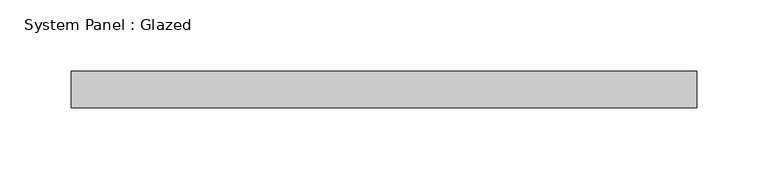
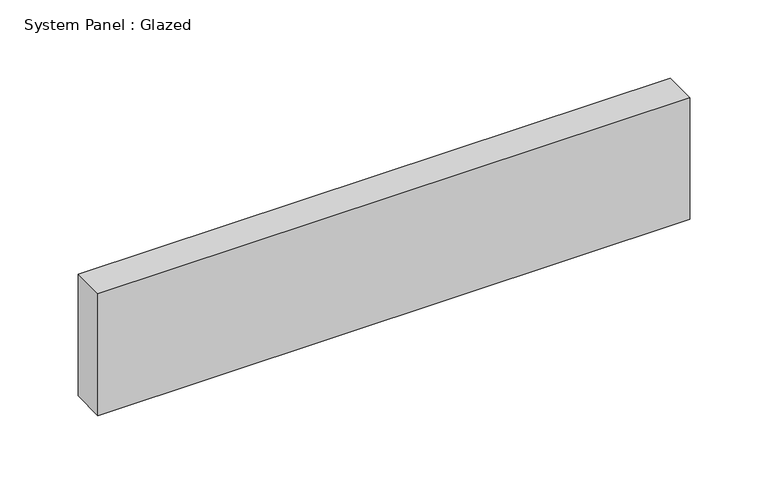
"""IFC4 building model written with IfcOpenShell, lengths in millimetres: plate geometry, System Panel : Glazed."""

from ifc_helpers import new_model, si_unit, origin, origin_with_axes, place, context, project, spatial, polyline, outline, extrude, source, transform, mapped, element, save


def system_panel_glazed_19038302(model_context):
    return source(origin(), model_context, "Body", "SweptSolid", [
        extrude(outline(polyline([(219.075, 19.05), (-219.075, 19.05), (-219.075, 44.45), (219.075, 44.45), (219.075, 19.05)])), origin_with_axes(), (0.0, 0.0, 1.0), 95.25),
    ])


if __name__ == "__main__":
    model = new_model("IFC4")
    model_context = context("Model", 3, world=origin())
    ifc_project = project(units=[si_unit("LENGTHUNIT", "METRE", prefix="MILLI")], contexts=[model_context])
    site = spatial("IfcSite", under=ifc_project)
    building = spatial("IfcBuilding", under=site)
    placement = place(None, origin())
    system_panel_glazed_shape = system_panel_glazed_19038302(model_context)
    element("IfcPlate", 1, ObjectType="System Panel : Glazed", at=placement, inside=building, context=model_context, shape_type="MappedRepresentation", body=[
        mapped(system_panel_glazed_shape, transform((0.0, 0.0, 0.0), x_axis=(1.0, 0.0, 0.0), y_axis=(0.0, 1.0, 0.0), z_axis=(0.0, 0.0, 1.0))),
    ])
    save(model, "model.ifc")

# Revit data of these elements
# Type "System Panel : Glazed"
#   Construction Type Id = "GSP4R"
#   Analytic Construction = "1/8 in Pilkington single glazing"
#   Visual Light Transmittance = 0.9
#   Solar Heat Gain Coefficient = 0.86
#   Heat Transfer Coefficient (U) = 1.18115 BTU/(h·ft²·°F)
#   Define Thermal Properties by = 1
# Element 1 (IfcPlate, "System Panel : Glazed")
#   Materials on its faces: "Glass"
# Materials
#   "Glass": class "Glass", colour RGB 0 128 192, transparency 0.75, Description = "Soda Lime Glass", Cost = 0
